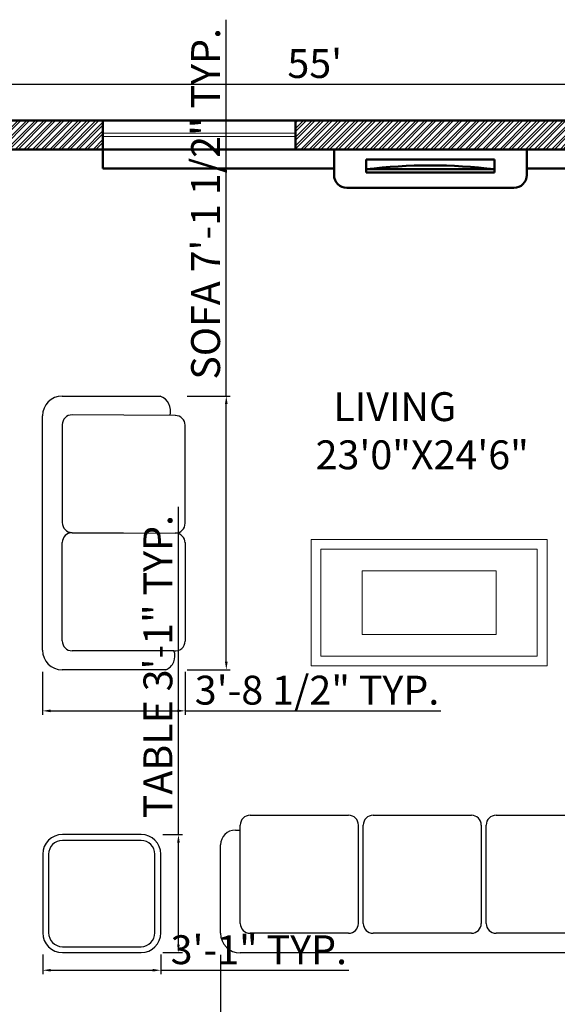
# Model space of a CAD drawing. Units: inches. Extents: x 3590 to 5167, y 65 to 1917.
# Tile 20 of 100: x 3884 to 4051, y 1531 to 1837. Entities that reach past the tile are written whole.
import ezdxf

# ---------------------------------------------------------------- set-up
doc = ezdxf.new("R2010")
doc.units = ezdxf.units.IN
for name, color, linetype, lineweight in [('A-ANNO-DIMS', 2, 'Continuous', 18), ('A-AREA-IDEN', 7, 'Continuous', 18), ('A-FURN', 21, 'Continuous', 18), ('A-GLAZ', 4, 'Continuous', 18), ('A-WALL', 7, 'Continuous', 50), ('A-WALL-PATT', 251, 'Continuous', 13)]:
    doc.layers.add(name, color=color, linetype=linetype, lineweight=lineweight)
doc.layers.add('M40-KOLTUKSUNGERI', color=136, linetype='Continuous')
doc.styles.get("Standard").update_dxf_attribs({"font": 'arial.ttf'})
doc.dimstyles.new('ISO-25', dxfattribs={"dimtxt": 9, "dimasz": 2.5, "dimexe": 1.25, "dimexo": 0.625, "dimtad": 1, "dimdec": 1, "dimlunit": 3, "dimtxsty": 'Standard', "dimcen": 2.5, "dimadec": 0, "dimazin": 0, "dimtfac": 1, "dimtdec": 1, "dimtmove": 0, "dimatfit": 3, "dimfxl": 1, "dimarcsym": 0})

# ---------------------------------------------------------------- blocks, each defined once
blk = doc.blocks.new('*D5')
at = {"layer": 'A-ANNO-DIMS', "color": 0, "lineweight": -2, "transparency": 16777216}
for p, q in [((3645.51, 1806.62), (3645.51, 1818.61)), ((3648.01, 1817.36), (4303.01, 1817.36)), ((4305.51, 1806.62), (4305.51, 1818.61))]:
    blk.add_line(p, q, dxfattribs=at)
at = {"layer": 'A-ANNO-DIMS', "color": 0, "transparency": 16777216}
for points in [[(3648.01, 1817.78), (3648.01, 1816.95), (3645.51, 1817.36)], [(4303.01, 1817.78), (4303.01, 1816.95), (4305.51, 1817.36)]]:
    blk.add_solid(points, dxfattribs=at)
at = {"layer": 'Defpoints', "color": 0, "transparency": 16777216}
for p in [(4305.51, 1817.36), (3645.51, 1806), (4305.51, 1806)]:
    blk.add_point(p, dxfattribs=at)
at = {"layer": 'A-ANNO-DIMS', "color": 0, "transparency": 16777216, "insert": (3975.51, 1822.57), "char_height": 9, "attachment_point": 5}
blk.add_mtext("55'", dxfattribs=at)
blk = doc.blocks.new('S1')
at = {"layer": 'M40-KOLTUKSUNGERI'}
for p, q in [((3.94, 27.4), (23.53, 27.4)), ((0, -23.47), (0, 23.47)), ((26.59, 23.52), (5.91, 23.65)), ((3.94, 21.68), (3.94, 2.06)), ((28.54, 1.93), (28.54, 21.55)), ((5.91, 0.09), (26.57, -0.04)), ((5.91, 0.03), (26.57, -0.04)), ((3.94, -21.63), (3.94, -1.94)), ((28.54, -1.94), (28.54, -21.67)), ((26.28, -23.6), (5.91, -23.6)), ((24.64, -27.4), (3.94, -27.4))]:
    blk.add_line(p, q, dxfattribs=at)
for centre, radius, start, end in [((3.94, 23.47), 3.94, 90, 180), ((22.44, 24.41), 3.19, 343.8468, 69.9238), ((5.91, 21.68), 1.97, 90, 180), ((26.57, 21.55), 1.97, 360, 90), ((5.91, 2.06), 1.97, 180, 270), ((5.91, -1.94), 1.97, 90, 180), ((26.57, 1.93), 1.97, 270, 0), ((26.57, -2.01), 1.97, 360, 90), ((5.91, -21.63), 1.97, 180, 270), ((26.6, -21.69), 1.94, 260.2828, 0.3826), ((3.94, -23.47), 3.94, 180, 270), ((23.58, -24.69), 2.91, 291.3314, 22.0931)]:
    blk.add_arc(centre, radius, start, end, dxfattribs=at)
blk = doc.blocks.new('S2')
at = {"layer": 'M40-KOLTUKSUNGERI'}
for p, q in [((-34.45, 27.56), (-14.76, 27.56)), ((-9.84, 27.56), (9.84, 27.56)), ((14.76, 27.56), (34.45, 27.56)), ((-37.4, 24.61), (-36.42, 24.61)), ((-36.42, 5.91), (-36.42, 25.59)), ((-12.8, 25.59), (-12.8, 5.91)), ((-11.81, 5.91), (-11.81, 25.59)), ((11.81, 25.59), (11.81, 5.91)), ((12.8, 5.91), (12.8, 25.59)), ((36.42, 25.59), (36.42, 5.91)), ((36.42, 24.61), (37.4, 24.61)), ((-40.35, 3.94), (-40.35, 21.65)), ((40.35, 21.65), (40.35, 3.94)), ((-14.76, 3.94), (-34.45, 3.94)), ((9.84, 3.94), (-9.84, 3.94)), ((34.45, 3.94), (14.76, 3.94)), ((36.42, 0), (-36.42, 0))]:
    blk.add_line(p, q, dxfattribs=at)
for centre, radius, start, end in [((-34.45, 25.59), 1.97, 90, 180), ((-14.76, 25.59), 1.97, 360, 90), ((-9.84, 25.59), 1.97, 90, 180), ((9.84, 25.59), 1.97, 360, 90), ((14.76, 25.59), 1.97, 90, 180), ((34.45, 25.59), 1.97, 360, 90), ((-37.4, 21.65), 2.95, 90, 180), ((37.4, 21.65), 2.95, 360, 90), ((-34.45, 5.91), 1.97, 180, 270), ((-14.76, 5.91), 1.97, 270, 0), ((-9.84, 5.91), 1.97, 180, 270), ((9.84, 5.91), 1.97, 270, 0), ((14.76, 5.91), 1.97, 180, 270), ((34.45, 5.91), 1.97, 270, 0), ((-36.42, 3.94), 3.94, 180, 270), ((36.42, 3.94), 3.94, 270, 0)]:
    blk.add_arc(centre, radius, start, end, dxfattribs=at)
blk = doc.blocks.new('T1')
at = {"layer": 'M40-KOLTUKSUNGERI'}
for p, q in [((4762.34, 1687.13), (4746.59, 1687.13)), ((4762.34, 1685.95), (4746.59, 1685.95)), ((4742.65, 1683.2), (4742.65, 1667.45)), ((4743.83, 1683.2), (4743.83, 1667.45)), ((4765.09, 1667.45), (4765.09, 1683.2)), ((4766.27, 1667.45), (4766.27, 1683.2)), ((4746.59, 1664.69), (4762.34, 1664.69)), ((4746.59, 1663.51), (4762.34, 1663.51))]:
    blk.add_line(p, q, dxfattribs=at)
for centre, radius, start, end in [((4746.59, 1683.2), 3.94, 90, 180), ((4746.59, 1683.2), 2.76, 90, 180), ((4762.34, 1683.2), 3.94, 360, 90), ((4762.34, 1683.2), 2.76, 360, 90), ((4746.59, 1667.45), 3.94, 180, 270), ((4746.59, 1667.45), 2.76, 180, 270), ((4762.34, 1667.45), 3.94, 270, 0), ((4762.34, 1667.45), 2.76, 270, 0)]:
    blk.add_arc(centre, radius, start, end, dxfattribs=at)
blk = doc.blocks.new('*D292')
at = {"layer": 'A-ANNO-DIMS', "color": 0, "lineweight": -2, "transparency": 16777216}
for p, q in [((3947.96, 1720.14), (3947.96, 1837.4)), ((3935.79, 1720.14), (3949.21, 1720.14)), ((3947.96, 1637.36), (3947.96, 1717.64)), ((3935.79, 1634.86), (3949.21, 1634.86))]:
    blk.add_line(p, q, dxfattribs=at)
at = {"layer": 'A-ANNO-DIMS', "color": 0, "transparency": 16777216}
for points in [[(3947.54, 1717.64), (3948.38, 1717.64), (3947.96, 1720.14)], [(3947.54, 1637.36), (3948.38, 1637.36), (3947.96, 1634.86)]]:
    blk.add_solid(points, dxfattribs=at)
at = {"layer": 'Defpoints', "color": 0, "transparency": 16777216}
for p in [(3935.17, 1720.14), (3947.96, 1720.14), (3935.17, 1634.86)]:
    blk.add_point(p, dxfattribs=at)
at = {"layer": 'A-ANNO-DIMS', "color": 0, "transparency": 16777216, "insert": (3942.68, 1780.02), "char_height": 9, "attachment_point": 5, "rotation": 90}
blk.add_mtext('SOFA 7\'-1 1/2" TYP.', dxfattribs=at)
blk = doc.blocks.new('*D293')
at = {"layer": 'A-ANNO-DIMS', "color": 0, "lineweight": -2, "transparency": 16777216}
for p, q in [((3890.75, 1634.24), (3890.75, 1620.82)), ((3935.17, 1634.24), (3935.17, 1620.82)), ((3893.25, 1622.07), (3932.67, 1622.07)), ((3935.17, 1622.07), (4014.74, 1622.07))]:
    blk.add_line(p, q, dxfattribs=at)
at = {"layer": 'A-ANNO-DIMS', "color": 0, "transparency": 16777216}
for points in [[(3893.25, 1622.49), (3893.25, 1621.65), (3890.75, 1622.07)], [(3932.67, 1622.49), (3932.67, 1621.65), (3935.17, 1622.07)]]:
    blk.add_solid(points, dxfattribs=at)
at = {"layer": 'Defpoints', "color": 0, "transparency": 16777216}
for p in [(3890.75, 1634.86), (3935.17, 1634.86), (3935.17, 1622.07)]:
    blk.add_point(p, dxfattribs=at)
at = {"layer": 'A-ANNO-DIMS', "color": 0, "transparency": 16777216, "insert": (3976.21, 1627.35), "char_height": 9, "attachment_point": 5}
blk.add_mtext('3\'-8 1/2" TYP.', dxfattribs=at)
blk = doc.blocks.new('*D294')
at = {"layer": 'A-ANNO-DIMS', "color": 0, "lineweight": -2, "transparency": 16777216}
for p, q in [((3946.19, 1546.03), (3946.19, 1526.56)), ((4071.76, 1546.03), (4071.76, 1526.56)), ((3948.69, 1527.81), (4069.26, 1527.81)), ((4071.76, 1527.81), (4243.57, 1527.81))]:
    blk.add_line(p, q, dxfattribs=at)
at = {"layer": 'A-ANNO-DIMS', "color": 0, "transparency": 16777216}
for points in [[(3948.69, 1528.23), (3948.69, 1527.4), (3946.19, 1527.81)], [(4069.26, 1528.23), (4069.26, 1527.4), (4071.76, 1527.81)]]:
    blk.add_solid(points, dxfattribs=at)
at = {"layer": 'Defpoints', "color": 0, "transparency": 16777216}
for p in [(3946.19, 1546.65), (4071.76, 1546.65), (4071.76, 1527.81)]:
    blk.add_point(p, dxfattribs=at)
at = {"layer": 'A-ANNO-DIMS', "color": 0, "transparency": 16777216, "insert": (4158.91, 1533.1), "char_height": 9, "attachment_point": 5}
blk.add_mtext('3-SEAT SOFA 10\'-5 1/2" TYP.', dxfattribs=at)
blk = doc.blocks.new('*D298')
at = {"layer": 'A-ANNO-DIMS', "color": 0, "lineweight": -2, "transparency": 16777216}
for p, q in [((3933.06, 1583.52), (3933.06, 1685.68)), ((3928.17, 1583.52), (3934.31, 1583.52)), ((3933.06, 1549.27), (3933.06, 1581.02)), ((3928.17, 1546.77), (3934.31, 1546.77))]:
    blk.add_line(p, q, dxfattribs=at)
at = {"layer": 'A-ANNO-DIMS', "color": 0, "transparency": 16777216}
for points in [[(3932.64, 1581.02), (3933.47, 1581.02), (3933.06, 1583.52)], [(3932.64, 1549.27), (3933.47, 1549.27), (3933.06, 1546.77)]]:
    blk.add_solid(points, dxfattribs=at)
at = {"layer": 'Defpoints', "color": 0, "transparency": 16777216}
for p in [(3927.54, 1583.52), (3933.06, 1583.52), (3927.54, 1546.77)]:
    blk.add_point(p, dxfattribs=at)
at = {"layer": 'A-ANNO-DIMS', "color": 0, "transparency": 16777216, "insert": (3927.83, 1635.85), "char_height": 9, "attachment_point": 5, "rotation": 90}
blk.add_mtext('TABLE 3\'-1" TYP.', dxfattribs=at)
blk = doc.blocks.new('*D299')
at = {"layer": 'A-ANNO-DIMS', "color": 0, "lineweight": -2, "transparency": 16777216}
for p, q in [((3890.79, 1546.14), (3890.79, 1540)), ((3927.54, 1546.14), (3927.54, 1540)), ((3893.29, 1541.25), (3925.04, 1541.25)), ((3927.54, 1541.25), (3986.15, 1541.25))]:
    blk.add_line(p, q, dxfattribs=at)
at = {"layer": 'A-ANNO-DIMS', "color": 0, "transparency": 16777216}
for points in [[(3893.29, 1541.67), (3893.29, 1540.84), (3890.79, 1541.25)], [(3925.04, 1541.67), (3925.04, 1540.84), (3927.54, 1541.25)]]:
    blk.add_solid(points, dxfattribs=at)
at = {"layer": 'Defpoints', "color": 0, "transparency": 16777216}
for p in [(3890.79, 1546.77), (3927.54, 1546.77), (3927.54, 1541.25)]:
    blk.add_point(p, dxfattribs=at)
at = {"layer": 'A-ANNO-DIMS', "color": 0, "transparency": 16777216, "insert": (3958.1, 1546.48), "char_height": 9, "attachment_point": 5}
blk.add_mtext('3\'-1" TYP.', dxfattribs=at)
blk = doc.blocks.new('*D318')
at = {"layer": 'A-ANNO-DIMS', "color": 0, "lineweight": -2, "transparency": 16777216}
for p, q in [((3874.41, 1620), (3874.41, 1738.94)), ((3869.64, 1620), (3875.66, 1620)), ((3874.41, 1586.5), (3874.41, 1617.5)), ((3869.64, 1584), (3875.66, 1584))]:
    blk.add_line(p, q, dxfattribs=at)
at = {"layer": 'A-ANNO-DIMS', "color": 0, "transparency": 16777216}
for points in [[(3874, 1617.5), (3874.83, 1617.5), (3874.41, 1620)], [(3874, 1586.5), (3874.83, 1586.5), (3874.41, 1584)]]:
    blk.add_solid(points, dxfattribs=at)
at = {"layer": 'Defpoints', "color": 0, "transparency": 16777216}
for p in [(3869.01, 1620), (3874.41, 1620), (3869.01, 1584)]:
    blk.add_point(p, dxfattribs=at)
at = {"layer": 'A-ANNO-DIMS', "color": 0, "transparency": 16777216, "insert": (3869.13, 1680.72), "char_height": 9, "attachment_point": 5, "rotation": 90}
blk.add_mtext('DOOR D3 3\'-0" TYP.', dxfattribs=at)

msp = doc.modelspace()

# ---------------------------------------------------------------- hatches: boundary and pattern name
at = {"layer": 'A-WALL-PATT', "transparency": 33554687}
h = msp.add_hatch(dxfattribs=at)
h.set_pattern_fill('ANSI32', color=256, scale=0.2)
h.paths.add_polyline_path([(3768.51, 1806), (3645.51, 1806), (3645.51, 1785), (3654.51, 1785), (3654.51, 1797), (3671.16, 1797), (3768.51, 1797)])
h.paths.add_polyline_path([(3909.51, 1806), (3816.51, 1806), (3816.51, 1797), (3864.51, 1797), (3864.51, 1791), (3873.51, 1791), (3873.51, 1797), (3909.51, 1797)])
h.paths.add_polyline_path([(4053.51, 1806), (3969.51, 1806), (3969.51, 1797), (4053.51, 1797)])
h.paths.add_polyline_path([(4215.51, 1806), (4113.51, 1806), (4113.51, 1797), (4206.51, 1797), (4206.51, 1791), (4215.51, 1791)])
h.paths.add_polyline_path([(3654.51, 1737), (3645.51, 1737), (3645.51, 1620), (3654.51, 1620), (3654.51, 1650), (3741.51, 1650), (3741.51, 1656), (3654.51, 1656)], flags=17)
h.paths.add_polyline_path([(3873.51, 1755), (3864.51, 1755), (3864.51, 1656), (3771.51, 1656), (3771.51, 1650), (3774.51, 1650), (3774.51, 1554), (3654.51, 1554), (3654.51, 1584), (3645.51, 1584), (3645.51, 1539), (3654.51, 1539), (3654.51, 1545), (3864.51, 1545), (3864.51, 1539), (3873.51, 1539), (3873.51, 1584), (3864.51, 1584), (3864.51, 1554), (3780.51, 1554), (3780.51, 1650), (3864.51, 1650), (3864.51, 1620), (3873.51, 1620)])
h.paths.add_polyline_path([(3654.51, 1491), (3645.51, 1491), (3645.51, 1326), (3810.51, 1326), (3810.51, 1335), (3809.96, 1335), (3654.51, 1335)])
h.paths.add_polyline_path([(3915.51, 1335), (3873.51, 1335), (3873.51, 1352.87), (3873.51, 1422), (3876.51, 1422), (3876.51, 1431), (3864.51, 1431), (3864.51, 1335), (3858.51, 1335), (3858.51, 1326), (3915.51, 1326)])
h.paths.add_polyline_path([(4028.01, 1335), (4002.51, 1335), (4002.51, 1503), (3981.51, 1503), (3981.51, 1494), (3993.51, 1494), (3993.51, 1431), (3921.51, 1431), (3921.51, 1494), (3933.51, 1494), (3933.51, 1503), (3864.51, 1503), (3864.51, 1494), (3912.51, 1494), (3912.51, 1431), (3906.51, 1431), (3906.51, 1422), (3993.51, 1422), (3993.51, 1335), (3951.51, 1335), (3951.51, 1326), (4028.01, 1326)])
h.paths.add_polyline_path([(4203.51, 1335), (4158.51, 1335), (4158.51, 1527), (4194.51, 1527), (4194.51, 1536), (4149.51, 1536), (4149.51, 1335), (4124.01, 1335), (4124.01, 1326), (4203.51, 1326)])
h.paths.add_polyline_path([(4305.51, 1566), (4296.51, 1566), (4296.51, 1536), (4278.64, 1536), (4260.51, 1536), (4260.51, 1527), (4296.51, 1527), (4296.51, 1521), (4305.51, 1521)])
h.paths.add_polyline_path([(4305.51, 1473), (4296.51, 1473), (4296.51, 1335), (4251.51, 1335), (4251.51, 1326), (4305.51, 1326)])
h.paths.add_polyline_path([(4305.51, 1677), (4215.51, 1677), (4215.51, 1743), (4206.51, 1743), (4206.51, 1677), (4149.51, 1677), (4149.51, 1668), (4296.51, 1668), (4296.51, 1638), (4305.51, 1638)])

# ---------------------------------------------------------------- linework, layer by layer
at = {"layer": 'A-FURN'}
for points in [[(3974.36, 1675.5), (4047.86, 1675.5), (4047.86, 1636.07), (3974.36, 1636.07)], [(3977.42, 1672.43), (4044.8, 1672.43), (4044.8, 1639.13), (3977.42, 1639.13)], [(3990.24, 1665.7), (4031.98, 1665.7), (4031.98, 1645.87), (3990.24, 1645.87)]]:
    msp.add_lwpolyline(points, close=True, dxfattribs=at)
at = {"layer": 'A-GLAZ'}
for p, q in [((3969.51, 1802), (3909.51, 1802)), ((3969.51, 1801), (3909.51, 1801))]:
    msp.add_line(p, q, dxfattribs=at)
at = {"layer": 'A-WALL'}
for p, q in [((3909.51, 1797), (3909.51, 1806)), ((3969.51, 1797), (3969.51, 1806)), ((3873.51, 1797), (4206.51, 1797)), ((3909.51, 1797), (3909.51, 1791)), ((3981.51, 1797), (3981.51, 1789)), ((4041.51, 1797), (4041.51, 1789)), ((3991.51, 1793.81), (3991.51, 1789.81)), ((3991.51, 1793.81), (4031.51, 1793.81)), ((4031.51, 1793.81), (4031.51, 1789.81)), ((3909.51, 1791), (3981.51, 1791)), ((4031.51, 1790.81), (3991.51, 1790.81)), ((4031.51, 1789.81), (3991.51, 1789.81)), ((4041.51, 1791), (4113.51, 1791)), ((3985.51, 1785), (4037.51, 1785))]:
    msp.add_line(p, q, dxfattribs=at)
msp.add_lwpolyline([(4305.51, 1677), (4305.51, 1326), (3645.51, 1326), (3645.51, 1806), (4215.51, 1806)], dxfattribs=at)
for centre, radius, start, end in [((4011.51, 1623.39), 168.61, 83.1879, 96.8121), ((3985.51, 1789), 4, 180, 270), ((4037.51, 1789), 4, 270, 0)]:
    msp.add_arc(centre, radius, start, end, dxfattribs=at)

# ---------------------------------------------------------------- block references
at = {"layer": 'A-FURN', "xscale": 1.555868517605225, "yscale": 1.555868517605225, "zscale": 1.555868517605225}
for name, p in [('S1', (3890.75, 1677.5)), ('S2', (4008.98, 1546.65)), ('T1', (-3488.15, -1041.44))]:
    msp.add_blockref(name, p, dxfattribs=at)

# ---------------------------------------------------------------- texts
at = {"layer": 'A-AREA-IDEN', "insert": (3975.77, 1721.34), "char_height": 9, "attachment_point": 1}
msp.add_mtext_dynamic_manual_height_columns('{\\fTimes New Roman|b0|i0|c0|p18;  LIVING\\P23\'0"X24\'6"}', width=67.3508, gutter_width=12.5, heights=[0], dxfattribs=at)

# ---------------------------------------------------------------- dimensions: what is measured, and where the dimension line sits
at = {"layer": 'A-ANNO-DIMS'}
for base, p1, p2, text, picture, middle in [((3947.96, 1720.14), (3935.17, 1634.86), (3935.17, 1720.14), 'SOFA <> TYP.', '*D292', (3942.68, 1780.02)), ((3874.41, 1620), (3869.01, 1584), (3869.01, 1620), 'DOOR D3 <> TYP.', '*D318', (3869.13, 1680.72)), ((3933.0571, 1583.5207), (3927.5442, 1546.7679), (3927.5442, 1583.5207), 'TABLE <> TYP.', '*D298', (3927.8339, 1635.851))]:
    dim = msp.add_linear_dim(base=base, p1=p1, p2=p2, angle=90, text=text, dimstyle='ISO-25', override={"dimdec": 1, "dimlfac": 1, "dimrnd": 0, "dimzin": 1, "dimdsep": 46, "dimlunit": 4, "dimfrac": 2}, dxfattribs=at)
    dim.commit()
    dim.dimension.update_dxf_attribs({"geometry": picture, "text_midpoint": middle})
dim = msp.add_linear_dim(base=(4305.51, 1817.36), p1=(3645.51, 1806), p2=(4305.51, 1806), dimstyle='ISO-25', override={"dimclrd": 0, "dimclre": 0, "dimclrt": 0}, dxfattribs=at)
dim.commit()
dim.dimension.update_dxf_attribs({"geometry": '*D5', "text_midpoint": (3975.51, 1822.57)})
for base, p1, p2, text, picture, middle in [((3935.17, 1622.07), (3890.75, 1634.86), (3935.17, 1634.86), '<> TYP.', '*D293', (3976.21, 1627.35)), ((4071.76, 1527.81), (3946.19, 1546.65), (4071.76, 1546.65), '3-SEAT SOFA <> TYP.', '*D294', (4158.91, 1533.1)), ((3927.5442, 1541.255), (3890.7914, 1546.7679), (3927.5442, 1546.7679), '<> TYP.', '*D299', (3958.0959, 1546.4782))]:
    dim = msp.add_linear_dim(base=base, p1=p1, p2=p2, text=text, dimstyle='ISO-25', override={"dimdec": 1, "dimlfac": 1, "dimrnd": 0, "dimzin": 1, "dimdsep": 46, "dimlunit": 4, "dimfrac": 2}, dxfattribs=at)
    dim.commit()
    dim.dimension.update_dxf_attribs({"geometry": picture, "text_midpoint": middle})

doc.saveas('drawing.dxf')
